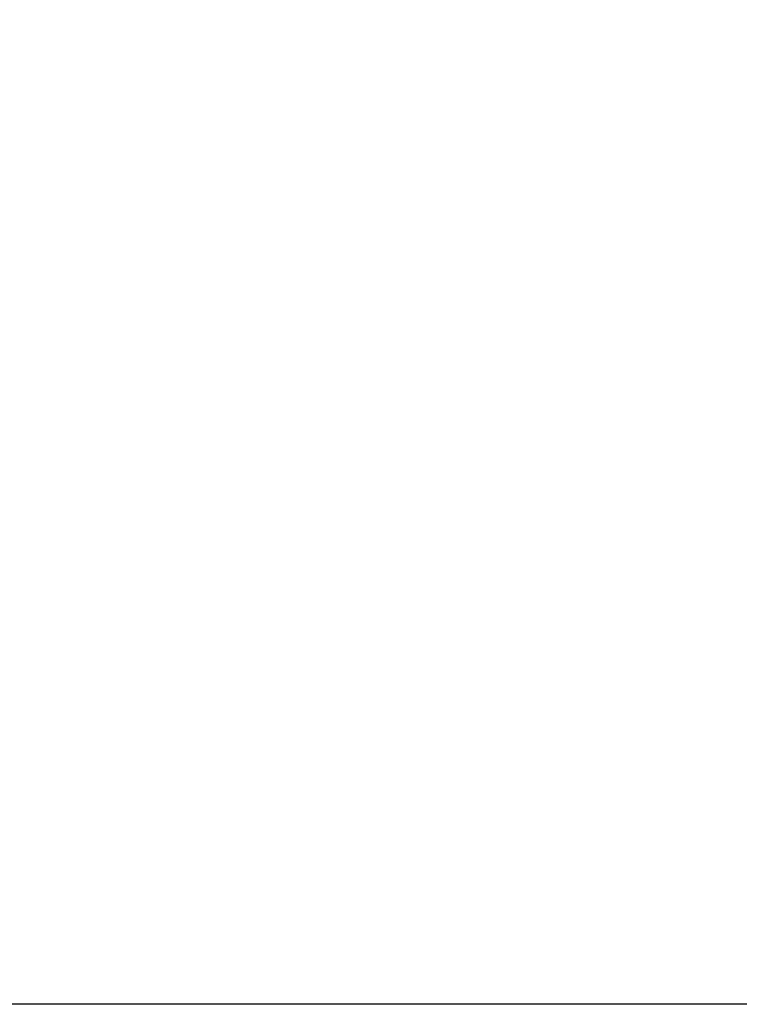
# Model space of a CAD drawing. Units: inches. Extents: x 2091 to 2899, y 967 to 2217.
# Tile 43 of 256: x 2193 to 2203, y 1100 to 1114. Entities that reach past the tile are written whole.
import ezdxf

# ---------------------------------------------------------------- set-up
doc = ezdxf.new("R2010")
doc.units = ezdxf.units.IN
doc.layers.add('A-ANNO-DIMS', color=2, linetype='Continuous', lineweight=18)
doc.styles.get("Standard").update_dxf_attribs({"font": 'arial.ttf'})
doc.dimstyles.new('ISO-25', dxfattribs={"dimtxt": 4, "dimasz": 4, "dimexe": 1.25, "dimexo": 0.625, "dimtad": 1, "dimdec": 0, "dimlunit": 3, "dimtxsty": 'Standard', "dimcen": 2.5, "dimadec": 0, "dimazin": 0, "dimtfac": 1, "dimtdec": 0, "dimtmove": 0, "dimatfit": 3, "dimfxl": 1, "dimarcsym": 0})

# ---------------------------------------------------------------- blocks, each defined once
blk = doc.blocks.new('*D91')
at = {"layer": 'A-ANNO-DIMS', "color": 0, "lineweight": -2, "transparency": 16777216}
for p, q in [((2211.651, 1152.247), (2098.311, 1152.247)), ((2099.561, 1103.919), (2099.561, 1148.247)), ((2211.519, 1099.919), (2098.311, 1099.919))]:
    blk.add_line(p, q, dxfattribs=at)
at = {"layer": 'A-ANNO-DIMS', "color": 0, "transparency": 16777216}
for points in [[(2098.895, 1148.247), (2100.228, 1148.247), (2099.561, 1152.247)], [(2098.895, 1103.919), (2100.228, 1103.919), (2099.561, 1099.919)]]:
    blk.add_solid(points, dxfattribs=at)
at = {"layer": 'Defpoints', "color": 0, "transparency": 16777216}
for p in [(2099.561, 1152.247), (2212.276, 1152.247), (2212.144, 1099.919)]:
    blk.add_point(p, dxfattribs=at)
at = {"layer": 'A-ANNO-DIMS', "color": 0, "transparency": 16777216, "insert": (2096.868, 1126.083), "char_height": 4, "attachment_point": 5, "rotation": 90}
blk.add_mtext('4\'-4 1/2"', dxfattribs=at)

msp = doc.modelspace()

# ---------------------------------------------------------------- dimensions: what is measured, and where the dimension line sits
at = {"layer": 'A-ANNO-DIMS'}
dim = msp.add_linear_dim(base=(2099.561, 1152.247), p1=(2212.144, 1099.919), p2=(2212.276, 1152.247), angle=90, dimstyle='ISO-25', override={"dimdec": 1, "dimlfac": 1, "dimrnd": 0, "dimzin": 1, "dimdsep": 46, "dimlunit": 4, "dimfrac": 2}, dxfattribs=at)
dim.commit()
dim.dimension.update_dxf_attribs({"geometry": '*D91', "text_midpoint": (2096.868, 1126.083)})

doc.saveas('drawing.dxf')
